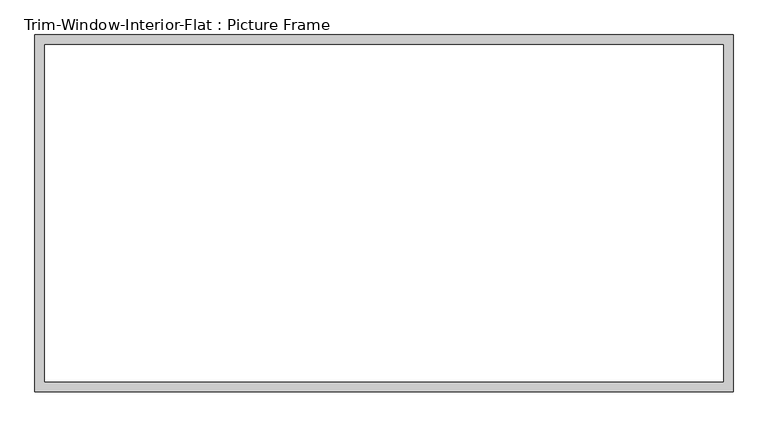
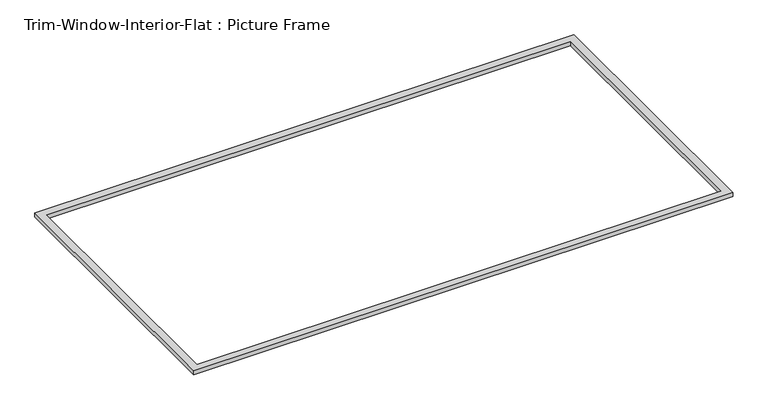
"""IFC4 building model written with IfcOpenShell, lengths in millimetres: proxy geometry, Trim-Window-Interior-Flat : Picture Frame."""

from ifc_helpers import new_model, si_unit, origin, origin_with_axes, place, context, project, spatial, polyline, outline, extrude, source, transform, mapped, element, save


def trim_window_interior_flat_picture_frame_cc79b2fe(model_context):
    return source(origin(), model_context, "Body", "SweptSolid", [
        extrude(outline(polyline([(2025.65, 44.45), (2025.65, -2025.65), (-2025.65, -2025.65), (-2025.65, 44.45), (2025.65, 44.45)]), holes=[polyline([(1968.5, -12.7), (-1968.5, -12.7), (-1968.5, -1968.5), (1968.5, -1968.5), (1968.5, -12.7)])]), origin_with_axes(), (0.0, 0.0, 1.0), 31.75),
    ])


if __name__ == "__main__":
    model = new_model("IFC4")
    model_context = context("Model", 3, world=origin())
    ifc_project = project(units=[si_unit("LENGTHUNIT", "METRE", prefix="MILLI")], contexts=[model_context])
    site = spatial("IfcSite", under=ifc_project)
    building = spatial("IfcBuilding", under=site)
    placement = place(None, origin())
    trim_window_interior_flat_picture_frame_shape = trim_window_interior_flat_picture_frame_cc79b2fe(model_context)
    element("IfcBuildingElementProxy", 1, Name="Trim-Window-Interior-Flat : Picture Frame", ObjectType="Trim-Window-Interior-Flat : Picture Frame", at=placement, inside=building, context=model_context, shape_type="MappedRepresentation", body=[
        mapped(trim_window_interior_flat_picture_frame_shape, transform((0.0, 0.0, 0.0), x_axis=(1.0, 0.0, 0.0), y_axis=(0.0, 1.0, 0.0), z_axis=(0.0, 0.0, 1.0))),
    ])
    save(model, "model.ifc")

# Revit data of these elements
# Type "Trim-Window-Interior-Flat : Picture Frame"
#   Trim Thickness_Picture Frame = 0.104167 ft
#   Trim Width = 0.1875 ft
#   Trim Thickness_with Sill = 0.0625 ft
#   Sill Thickness = 0.104167 ft
#   Opening Width [instance default] = 2 ft
#   Opening Height [instance default] = 3 ft
#   Default Elevation = 4 ft
#   Sill = no
#   Picture Frame = yes
#   Trim Material [instance default] = none
# Element 1 (IfcBuildingElementProxy, "Trim-Window-Interior-Flat : Picture Frame")
#   Opening Width = 13 ft
#   Opening Height = 6.5 ft
#   Trim Material = Wood - Stained
#   Materials on its faces: "Wood - Stained"
# Materials
#   "Wood - Stained": class "Wood", colour RGB 224 178 126, transparency 0, Cost = 0
